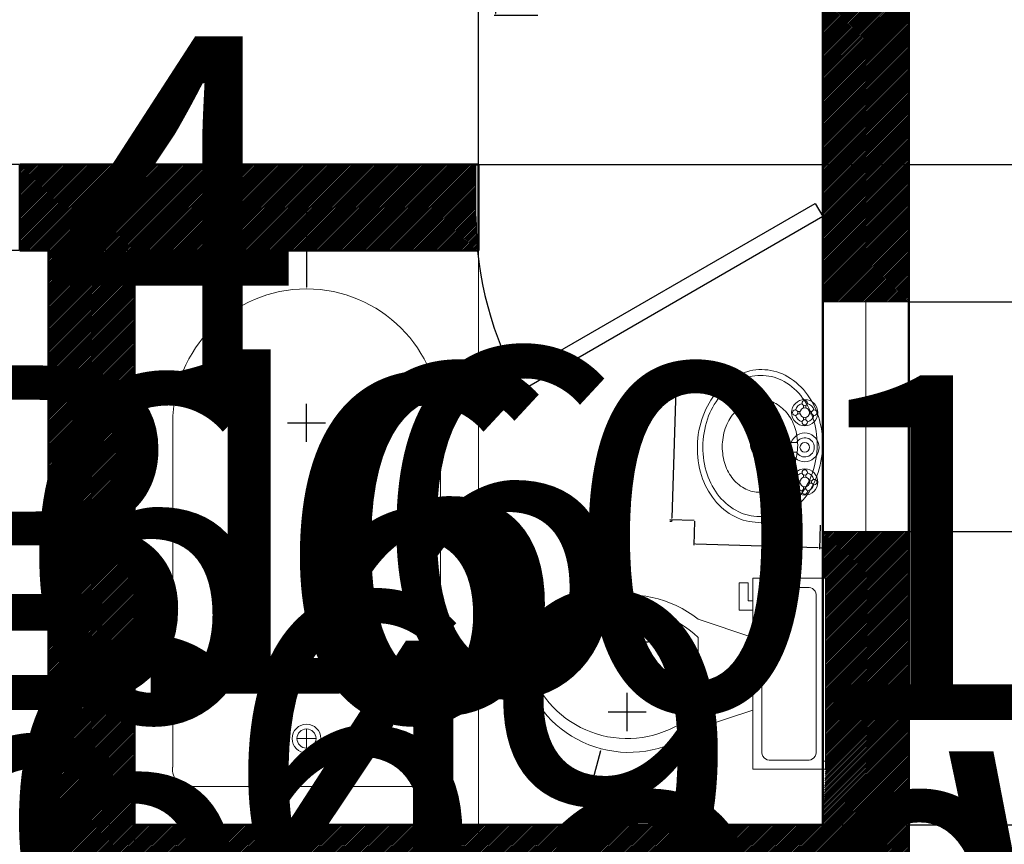
# Model space of a CAD drawing. Units: inches. Extents: x 1173 to 2157, y 515 to 1129.
# Tile 8 of 13: x 1578 to 1681, y 862 to 948. Entities that reach past the tile are written whole.
import ezdxf

# ---------------------------------------------------------------- set-up
doc = ezdxf.new("R2010")
doc.units = ezdxf.units.IN
doc.header["$MEASUREMENT"] = 0
for name, color, linetype, lineweight in [('A-ANNO-DIMS', 2, 'Continuous', 18), ('A-DOOR', 3, 'Continuous', 25), ('A-FLOR-FIXT', 9, 'Continuous', 18), ('A-GLAZ', 4, 'Continuous', 18), ('A-WALL', 7, 'Continuous', 50)]:
    doc.layers.add(name, color=color, linetype=linetype, lineweight=lineweight)
doc.layers.add('A-WALL-PATT', color=22, linetype='Continuous', lineweight=13, true_color=0xca4b0c)
doc.styles.get("Standard").update_dxf_attribs({"font": 'arial.ttf'})
doc.dimstyles.get("Standard").update_dxf_attribs({"dimtxt": 36, "dimasz": 0.18, "dimexe": 0.18, "dimexo": 0.0625, "dimgap": 0.09, "dimtad": 0, "dimtih": 1, "dimtoh": 1, "dimdec": 0, "dimrnd": 72, "dimzin": 0, "dimdsep": 46, "dimlunit": 3, "dimtxsty": 'Standard', "dimcen": 2, "dimadec": 0, "dimazin": 0, "dimtfac": 1, "dimtdec": 0, "dimtofl": 0, "dimtmove": 0, "dimatfit": 3, "dimfxl": 1, "dimtolj": 1, "dimtzin": 0, "dimarcsym": 0})

# ---------------------------------------------------------------- blocks, each defined once
blk = doc.blocks.new('*U23')
for p, q in [((-40, 0), (-40, 6)), ((0, 0), (0, 6))]:
    blk.add_line(p, q)
blk.add_lwpolyline([(0, 0), (-34.64, -20), (-35.52, -18.48), (-0.88, 1.52)], close=True)
blk.add_arc((0, 0), 40, 180, 210)
blk = doc.blocks.new('Bath Tub - 26 x 60 in.')
for p, q in [((9, -17), (9, -19)), ((8, -18), (10, -18))]:
    blk.add_line(p, q)
blk.add_lwpolyline([(0, -36), (0, 0), (60, 0), (60, -36)], close=True)
for points in [[(6, -4), (42, -4)], [(4, -30), (4, -6)], [(42, -32), (6, -32)]]:
    blk.add_lwpolyline(points)
for radius in [1.5, 1]:
    blk.add_circle((9, -18), radius)
for centre, radius, start, end in [((5.75, -5.75), 1.77, 81.8699, 188.1301), ((42, -18), 14, 270, 90), ((5.75, -30.25), 1.77, 171.8699, 278.1301)]:
    blk.add_arc(centre, radius, start, end)
blk = doc.blocks.new('Toilet - top')
for p, q in [((9.5, -6), (9.5, -2)), ((-10, -8.5), (-8, -8.5)), ((-10, -9.5), (-10, -8.5)), ((-8, -8.5), (-8, -8)), ((-7, -8), (-7, -9.5)), ((-4, -8), (-6, -14)), ((4, -8), (6, -14)), ((-7, -9.5), (-10, -9.5)), ((4, -14), (-4, -14))]:
    blk.add_line(p, q)
blk.add_lwpolyline([(10.5, -8), (10.5, 0), (-10.5, 0), (-10.5, -8)], close=True)
for points in [[(8.5, -1), (-8.5, -1)], [(-9.5, -2), (-9.5, -6)], [(-8.5, -7), (8.5, -7)]]:
    blk.add_lwpolyline(points)
for centre, radius, start, end in [((-8.62, -1.88), 0.884, 81.8699, 188.1301), ((8.62, -1.88), 0.884, 351.8699, 98.1301), ((-8.62, -6.12), 0.884, 171.8699, 278.1301), ((8.62, -6.12), 0.884, 261.8699, 8.1301), ((3.52, -21.58), 12.17, 141.4691, 247.9714), ((4.2, -21.82), 11.33, 136.3677, 238.9468), ((-3.52, -21.58), 12.17, 292.0284, 38.5307), ((-4.2, -21.82), 11.33, 301.053, 43.6321), ((0, -27.88), 4, 245.7318, 294.2682), ((0, -29), 4, 254.8605, 285.1395)]:
    blk.add_arc(centre, radius, start, end)
blk = doc.blocks.new('Sink - Oval top')
for p, q in [((-1, 0), (1, 0)), ((0, 1), (0, -1))]:
    blk.add_line(p, q)
for points in [[(-12.23, 0.39, 0.117634), (-11.46, -3.36, 0.104469), (-8.88, -6.8, 0.090016), (-5.08, -9.07, 0.08192), (-0.32, -10.02, 0.08192), (4.49, -9.38, 0.090016), (8.42, -7.36, 0.104469), (11.22, -4.09, 0.117634), (12.23, -0.39, 0.117634), (11.46, 3.36, 0.104469), (8.88, 6.8, 0.090016), (5.08, 9.07, 0.08192), (0.32, 10.02, 0.08192), (-4.49, 9.38, 0.090016), (-8.42, 7.36, 0.104469), (-11.22, 4.09, 0.117634)], [(-11.29, 0.16, 0.118622), (-10.52, -3.25, 0.104678), (-8.07, -6.36, 0.089562), (-4.54, -8.37, 0.081185), (-0.13, -9.15, 0.081185), (4.3, -8.49, 0.089562), (7.89, -6.58, 0.104678), (10.42, -3.55, 0.118622), (11.29, -0.16, 0.118622), (10.52, 3.25, 0.104678), (8.07, 6.36, 0.089562), (4.54, 8.37, 0.081185), (0.13, 9.15, 0.081185), (-4.3, 8.49, 0.089562), (-7.89, 6.58, 0.104678), (-10.42, 3.55, 0.118622)], [(-7.42, 0.08, 0.118283), (-6.91, -2.17, 0.104607), (-5.29, -4.21, 0.089718), (-2.97, -5.53, 0.081436), (-0.07, -6.04, 0.081436), (2.84, -5.59, 0.089718), (5.2, -4.33, 0.104607), (6.86, -2.32, 0.118283), (7.42, -0.08, 0.118283), (6.91, 2.17, 0.104607), (5.29, 4.21, 0.089718), (2.97, 5.53, 0.081436), (0.07, 6.04, 0.081436), (-2.84, 5.59, 0.089718), (-5.2, 4.33, 0.104607), (-6.86, 2.32, 0.118283)]]:
    blk.add_lwpolyline(points, format="xyb", close=True)
for radius in [1.5, 1]:
    blk.add_circle((0, 0), radius)
blk = doc.blocks.new('Faucet - Bathroom top')
for p, q in [((-4.107, 0.125), (-4.375, 0.125)), ((-3.75, 0.4788), (-3.75, 0.75)), ((-3.5, 0.482), (-3.5, 0.75)), ((-3.1461, 0.125), (-2.875, 0.125)), ((3.143, 0.125), (2.875, 0.125)), ((3.5, 0.4788), (3.5, 0.75)), ((3.75, 0.482), (3.75, 0.75)), ((4.1039, 0.125), (4.375, 0.125)), ((-4.1039, -0.125), (-4.375, -0.125)), ((-3.75, -0.4821), (-3.75, -0.75)), ((-3.5, -0.4789), (-3.5, -0.75)), ((-3.143, -0.125), (-2.875, -0.125)), ((-0.5, -0.8639), (-0.5, -4.5)), ((0.5, -4.5), (0.5, -0.8631)), ((3.1461, -0.125), (2.875, -0.125)), ((3.5, -0.4821), (3.5, -0.75)), ((3.75, -0.4789), (3.75, -0.75)), ((4.107, -0.125), (4.375, -0.125))]:
    blk.add_line(p, q)
for centre, radius in [((-3.625, 0), 1.375), ((-3.625, 1), 0.2795), ((3.625, 0), 1.375), ((3.625, 1), 0.2795), ((-4.625, 0), 0.2795), ((-3.625, 0), 0.5), ((-2.625, 0), 0.2795), ((0, 0), 0.5), ((2.625, 0), 0.2795), ((3.625, 0), 0.5), ((4.625, 0), 0.2795), ((-3.625, -1), 0.2795), ((3.625, -1), 0.2795)]:
    blk.add_circle(centre, radius)
for centre, radius, start, end in [((0, 0), 1.5, 289.6514, 250.3603), ((-3.625, 0), 1, 105.2407, 164.2093), ((-3.625, 0), 1, 16.44125, 74.07887), ((0, 0), 1, 300.3431, 239.7554), ((3.625, 0), 1, 106.12, 164.0884), ((3.625, 0), 1, 16.23422, 73.90469), ((-3.625, 0), 1, 196.2342, 253.9047), ((-3.625, 0), 1, 286.12, 344.0884), ((3.625, 0), 1, 196.4413, 254.0789), ((3.625, 0), 1, 285.2407, 344.2093), ((0, -4.5), 0.5, 180, 0)]:
    blk.add_arc(centre, radius, start, end)
blk = doc.blocks.new('*D28')
at = {"layer": 'A-ANNO-DIMS', "color": 0, "lineweight": -2, "transparency": 16777216}
for p, q in [((1581.66, 978.31), (1581.66, 966.19)), ((1661.66, 978.31), (1661.66, 966.19)), ((1581.84, 966.37), (1661.48, 966.37)), ((1661.66, 966.37), (1661.84, 966.37))]:
    blk.add_line(p, q, dxfattribs=at)
at = {"layer": 'A-ANNO-DIMS', "color": 0, "transparency": 16777216}
for points in [[(1581.84, 966.4), (1581.84, 966.34), (1581.66, 966.37)], [(1661.48, 966.4), (1661.48, 966.34), (1661.66, 966.37)]]:
    blk.add_solid(points, dxfattribs=at)
at = {"layer": 'Defpoints', "color": 0, "transparency": 16777216}
for p in [(1581.66, 978.37), (1661.66, 978.37), (1661.66, 966.37)]:
    blk.add_point(p, dxfattribs=at)
at = {"layer": 'A-ANNO-DIMS', "color": 0, "transparency": 16777216, "insert": (1904.61, 966.37), "char_height": 36, "attachment_point": 5}
blk.add_mtext('\\A1;QUEEN BED 80 TYP.', dxfattribs=at)
blk = doc.blocks.new('*D34')
at = {"layer": 'A-ANNO-DIMS', "color": 0, "lineweight": -2, "transparency": 16777216}
for p, q in [((1631.9, 978.41), (1631.9, 982.97)), ((1632.08, 982.79), (1661.32, 982.79)), ((1661.5, 978.41), (1661.5, 982.97)), ((1661.5, 982.79), (1661.68, 982.79))]:
    blk.add_line(p, q, dxfattribs=at)
at = {"layer": 'A-ANNO-DIMS', "color": 0, "transparency": 16777216}
for points in [[(1632.08, 982.82), (1632.08, 982.76), (1631.9, 982.79)], [(1661.32, 982.82), (1661.32, 982.76), (1661.5, 982.79)]]:
    blk.add_solid(points, dxfattribs=at)
at = {"layer": 'Defpoints', "color": 0, "transparency": 16777216}
for p in [(1661.5, 982.79), (1631.9, 978.35), (1661.5, 978.35)]:
    blk.add_point(p, dxfattribs=at)
at = {"layer": 'A-ANNO-DIMS', "color": 0, "transparency": 16777216, "insert": (1918.96, 982.79), "char_height": 36, "attachment_point": 5}
blk.add_mtext('\\A1;NIGHTSTAND 30 TYP.', dxfattribs=at)
blk = doc.blocks.new('*D35')
at = {"layer": 'A-ANNO-DIMS', "color": 0, "lineweight": -2, "transparency": 16777216}
for p, q in [((1631.84, 978.35), (1627.28, 978.35)), ((1627.46, 978.35), (1627.46, 978.53)), ((1627.46, 978.53), (1627.64, 978.53)), ((1627.46, 949.05), (1627.46, 978.17)), ((1631.84, 948.87), (1627.28, 948.87))]:
    blk.add_line(p, q, dxfattribs=at)
at = {"layer": 'A-ANNO-DIMS', "color": 0, "transparency": 16777216}
for points in [[(1627.43, 978.17), (1627.49, 978.17), (1627.46, 978.35)], [(1627.43, 949.05), (1627.49, 949.05), (1627.46, 948.87)]]:
    blk.add_solid(points, dxfattribs=at)
at = {"layer": 'Defpoints', "color": 0, "transparency": 16777216}
for p in [(1627.46, 978.35), (1631.9, 978.35), (1631.9, 948.87)]:
    blk.add_point(p, dxfattribs=at)
at = {"layer": 'A-ANNO-DIMS', "color": 0, "transparency": 16777216, "insert": (1715.66, 978.53), "char_height": 36, "attachment_point": 5}
blk.add_mtext('\\A1;29 TYP.', dxfattribs=at)
blk = doc.blocks.new('*D36')
at = {"layer": 'A-ANNO-DIMS', "color": 0, "lineweight": -2, "transparency": 16777216}
for p, q in [((1497.87, 905.02), (1487.37, 905.02)), ((1487.55, 904.84), (1487.55, 889.09)), ((1487.55, 835.93), (1487.55, 851.68)), ((1497.87, 835.75), (1487.37, 835.75))]:
    blk.add_line(p, q, dxfattribs=at)
at = {"layer": 'A-ANNO-DIMS', "color": 0, "transparency": 16777216}
for points in [[(1487.52, 904.84), (1487.58, 904.84), (1487.55, 905.02)], [(1487.52, 835.93), (1487.58, 835.93), (1487.55, 835.75)]]:
    blk.add_solid(points, dxfattribs=at)
at = {"layer": 'Defpoints', "color": 0, "transparency": 16777216}
for p in [(1497.94, 905.02), (1487.55, 835.75), (1497.94, 835.75)]:
    blk.add_point(p, dxfattribs=at)
at = {"layer": 'A-ANNO-DIMS', "color": 0, "transparency": 16777216, "insert": (1487.55, 870.38), "char_height": 36, "attachment_point": 5}
blk.add_mtext('\\A1;DINING SET 69', dxfattribs=at)
blk = doc.blocks.new('*D38')
at = {"layer": 'A-ANNO-DIMS', "color": 0, "lineweight": -2, "transparency": 16777216}
for p, q in [((1471.69, 862.7), (1478.04, 862.7)), ((1477.86, 862.52), (1477.86, 860.65)), ((1477.86, 821.35), (1477.86, 823.22)), ((1471.69, 821.17), (1478.04, 821.17))]:
    blk.add_line(p, q, dxfattribs=at)
at = {"layer": 'A-ANNO-DIMS', "color": 0, "transparency": 16777216}
for points in [[(1477.83, 862.52), (1477.89, 862.52), (1477.86, 862.7)], [(1477.83, 821.35), (1477.89, 821.35), (1477.86, 821.17)]]:
    blk.add_solid(points, dxfattribs=at)
at = {"layer": 'Defpoints', "color": 0, "transparency": 16777216}
for p in [(1471.63, 862.7), (1477.86, 862.7), (1471.63, 821.17)]:
    blk.add_point(p, dxfattribs=at)
at = {"layer": 'A-ANNO-DIMS', "color": 0, "transparency": 16777216, "insert": (1477.86, 841.93), "char_height": 36, "attachment_point": 5}
blk.add_mtext('\\A1;COFFEE TABLE 42', dxfattribs=at)
blk = doc.blocks.new('*D40')
at = {"layer": 'A-ANNO-DIMS', "color": 0, "lineweight": -2, "transparency": 16777216}
for p, q in [((1422.73, 872.86), (1431.84, 872.86)), ((1431.66, 872.68), (1431.66, 861.58)), ((1431.66, 813.04), (1431.66, 824.15)), ((1422.73, 812.86), (1431.84, 812.86))]:
    blk.add_line(p, q, dxfattribs=at)
at = {"layer": 'A-ANNO-DIMS', "color": 0, "transparency": 16777216}
for points in [[(1431.63, 872.68), (1431.69, 872.68), (1431.66, 872.86)], [(1431.63, 813.04), (1431.69, 813.04), (1431.66, 812.86)]]:
    blk.add_solid(points, dxfattribs=at)
at = {"layer": 'Defpoints', "color": 0, "transparency": 16777216}
for p in [(1422.66, 872.86), (1431.66, 872.86), (1422.66, 812.86)]:
    blk.add_point(p, dxfattribs=at)
at = {"layer": 'A-ANNO-DIMS', "color": 0, "transparency": 16777216, "insert": (1431.66, 842.86), "char_height": 36, "attachment_point": 5}
blk.add_mtext('\\A1;LOVESEAT 60', dxfattribs=at)
blk = doc.blocks.new('*D44')
at = {"layer": 'A-ANNO-DIMS', "color": 0, "lineweight": -2, "transparency": 16777216}
for p, q in [((1630.26, 849.3), (1630.26, 854.13)), ((1630.44, 853.95), (1661.48, 853.95)), ((1661.66, 849.3), (1661.66, 854.13)), ((1661.66, 853.95), (1661.84, 853.95))]:
    blk.add_line(p, q, dxfattribs=at)
at = {"layer": 'A-ANNO-DIMS', "color": 0, "transparency": 16777216}
for points in [[(1630.44, 853.98), (1630.44, 853.92), (1630.26, 853.95)], [(1661.48, 853.98), (1661.48, 853.92), (1661.66, 853.95)]]:
    blk.add_solid(points, dxfattribs=at)
at = {"layer": 'Defpoints', "color": 0, "transparency": 16777216}
for p in [(1661.66, 853.95), (1630.26, 849.24), (1661.66, 849.24)]:
    blk.add_point(p, dxfattribs=at)
at = {"layer": 'A-ANNO-DIMS', "color": 0, "transparency": 16777216, "insert": (1799.17, 853.95), "char_height": 36, "attachment_point": 5}
blk.add_mtext('\\A1;WC 31 TYP.', dxfattribs=at)
blk = doc.blocks.new('*D45')
at = {"layer": 'A-ANNO-DIMS', "color": 0, "lineweight": -2, "transparency": 16777216}
for p, q in [((1630.2, 849.24), (1625.37, 849.24)), ((1625.55, 849.24), (1625.55, 849.42)), ((1625.55, 849.42), (1625.73, 849.42)), ((1625.55, 829.46), (1625.55, 849.06)), ((1630.2, 829.28), (1625.37, 829.28))]:
    blk.add_line(p, q, dxfattribs=at)
at = {"layer": 'A-ANNO-DIMS', "color": 0, "transparency": 16777216}
for points in [[(1625.52, 849.06), (1625.58, 849.06), (1625.55, 849.24)], [(1625.52, 829.46), (1625.58, 829.46), (1625.55, 829.28)]]:
    blk.add_solid(points, dxfattribs=at)
at = {"layer": 'Defpoints', "color": 0, "transparency": 16777216}
for p in [(1625.55, 849.24), (1630.26, 849.24), (1630.26, 829.28)]:
    blk.add_point(p, dxfattribs=at)
at = {"layer": 'A-ANNO-DIMS', "color": 0, "transparency": 16777216, "insert": (1713.74, 849.42), "char_height": 36, "attachment_point": 5}
blk.add_mtext('\\A1;20 TYP.', dxfattribs=at)
blk = doc.blocks.new('*D46')
at = {"layer": 'A-ANNO-DIMS', "color": 0, "lineweight": -2, "transparency": 16777216}
for p, q in [((1646.37, 911.98), (1645.86, 896.32)), ((1648.72, 912.09), (1646.2, 912.17)), ((1645.85, 895.96), (1645.67, 895.96)), ((1648.2, 896.07), (1645.68, 896.15)), ((1645.86, 896.14), (1645.85, 895.96))]:
    blk.add_line(p, q, dxfattribs=at)
at = {"layer": 'A-ANNO-DIMS', "color": 0, "transparency": 16777216}
for points in [[(1646.34, 911.99), (1646.4, 911.98), (1646.38, 912.16)], [(1645.83, 896.32), (1645.89, 896.32), (1645.86, 896.14)]]:
    blk.add_solid(points, dxfattribs=at)
at = {"layer": 'Defpoints', "color": 0, "transparency": 16777216}
for p in [(1648.78, 912.09), (1645.86, 896.14), (1648.26, 896.06)]:
    blk.add_point(p, dxfattribs=at)
at = {"layer": 'A-ANNO-DIMS', "color": 0, "transparency": 16777216, "insert": (1538.16, 895.96), "char_height": 36, "attachment_point": 5}
blk.add_mtext('\\A1;BASIN 16', dxfattribs=at)
blk = doc.blocks.new('*D47')
at = {"layer": 'A-ANNO-DIMS', "color": 0, "lineweight": -2, "transparency": 16777216}
for p, q in [((1648.26, 896), (1648.18, 893.48)), ((1661.4, 895.58), (1661.32, 893.06)), ((1648.36, 893.65), (1661.15, 893.24)), ((1661.33, 893.24), (1661.51, 893.23))]:
    blk.add_line(p, q, dxfattribs=at)
at = {"layer": 'A-ANNO-DIMS', "color": 0, "transparency": 16777216}
for points in [[(1648.37, 893.68), (1648.36, 893.62), (1648.18, 893.66)], [(1661.15, 893.27), (1661.15, 893.21), (1661.33, 893.24)]]:
    blk.add_solid(points, dxfattribs=at)
at = {"layer": 'Defpoints', "color": 0, "transparency": 16777216}
for p in [(1648.26, 896.06), (1661.4, 895.64), (1661.33, 893.24)]:
    blk.add_point(p, dxfattribs=at)
at = {"layer": 'A-ANNO-DIMS', "color": 0, "transparency": 16777216, "insert": (1685.69, 893.23), "char_height": 36, "attachment_point": 5}
blk.add_mtext('\\A1;13', dxfattribs=at)
blk = doc.blocks.new('*D48')
at = {"layer": 'A-ANNO-DIMS', "color": 0, "lineweight": -2, "transparency": 16777216}
for p, q in [((1592.53, 826.46), (1592.35, 826.47)), ((1592.38, 821.85), (1592.54, 826.64)), ((1623.53, 825.46), (1592.71, 826.46)), ((1623.56, 820.84), (1623.71, 825.64))]:
    blk.add_line(p, q, dxfattribs=at)
at = {"layer": 'A-ANNO-DIMS', "color": 0, "transparency": 16777216}
for points in [[(1592.71, 826.49), (1592.71, 826.43), (1592.53, 826.46)], [(1623.53, 825.49), (1623.53, 825.43), (1623.71, 825.46)]]:
    blk.add_solid(points, dxfattribs=at)
at = {"layer": 'Defpoints', "color": 0, "transparency": 16777216}
for p in [(1592.53, 826.46), (1592.38, 821.79), (1623.56, 820.78)]:
    blk.add_point(p, dxfattribs=at)
at = {"layer": 'A-ANNO-DIMS', "color": 0, "transparency": 16777216, "insert": (1488.3, 826.47), "char_height": 36, "attachment_point": 5}
blk.add_mtext('\\A1;BASIN 31', dxfattribs=at)
blk = doc.blocks.new('*D50')
at = {"layer": 'A-ANNO-DIMS', "color": 0, "lineweight": -2, "transparency": 16777216}
for p, q in [((1603.33, 798.21), (1603.33, 796.59)), ((1613.33, 798.21), (1613.33, 796.59)), ((1603.33, 796.77), (1603.15, 796.77)), ((1613.15, 796.77), (1603.51, 796.77))]:
    blk.add_line(p, q, dxfattribs=at)
at = {"layer": 'A-ANNO-DIMS', "color": 0, "transparency": 16777216}
for points in [[(1603.51, 796.8), (1603.51, 796.74), (1603.33, 796.77)], [(1613.15, 796.8), (1613.15, 796.74), (1613.33, 796.77)]]:
    blk.add_solid(points, dxfattribs=at)
at = {"layer": 'Defpoints', "color": 0, "transparency": 16777216}
for p in [(1603.33, 798.27), (1613.33, 798.27), (1603.33, 796.77)]:
    blk.add_point(p, dxfattribs=at)
at = {"layer": 'A-ANNO-DIMS', "color": 0, "transparency": 16777216, "insert": (1377.9, 796.77), "char_height": 36, "attachment_point": 5}
blk.add_mtext('\\A1;BASIN TAP 10 TYP.', dxfattribs=at)
blk = doc.blocks.new('*D52')
at = {"layer": 'A-ANNO-DIMS', "color": 0, "lineweight": -2, "transparency": 16777216}
for p, q in [((1589.6, 924.28), (1580.48, 924.28)), ((1580.66, 924.1), (1580.66, 912.75)), ((1580.66, 864.46), (1580.66, 875.81)), ((1589.6, 864.28), (1580.48, 864.28))]:
    blk.add_line(p, q, dxfattribs=at)
at = {"layer": 'A-ANNO-DIMS', "color": 0, "transparency": 16777216}
for points in [[(1580.63, 924.1), (1580.69, 924.1), (1580.66, 924.28)], [(1580.63, 864.46), (1580.69, 864.46), (1580.66, 864.28)]]:
    blk.add_solid(points, dxfattribs=at)
at = {"layer": 'Defpoints', "color": 0, "transparency": 16777216}
for p in [(1580.66, 924.28), (1589.66, 924.28), (1589.66, 864.28)]:
    blk.add_point(p, dxfattribs=at)
at = {"layer": 'A-ANNO-DIMS', "color": 0, "transparency": 16777216, "insert": (1580.66, 894.28), "char_height": 36, "attachment_point": 5}
blk.add_mtext('\\A1;TUB 60', dxfattribs=at)
blk = doc.blocks.new('*D53')
at = {"layer": 'A-ANNO-DIMS', "color": 0, "lineweight": -2, "transparency": 16777216}
for p, q in [((1589.66, 864.22), (1589.66, 855.1)), ((1625.66, 864.22), (1625.66, 855.1)), ((1589.66, 855.28), (1589.48, 855.28)), ((1625.48, 855.28), (1589.84, 855.28))]:
    blk.add_line(p, q, dxfattribs=at)
at = {"layer": 'A-ANNO-DIMS', "color": 0, "transparency": 16777216}
for points in [[(1589.84, 855.31), (1589.84, 855.25), (1589.66, 855.28)], [(1625.48, 855.31), (1625.48, 855.25), (1625.66, 855.28)]]:
    blk.add_solid(points, dxfattribs=at)
at = {"layer": 'Defpoints', "color": 0, "transparency": 16777216}
for p in [(1589.66, 864.28), (1625.66, 864.28), (1589.66, 855.28)]:
    blk.add_point(p, dxfattribs=at)
at = {"layer": 'A-ANNO-DIMS', "color": 0, "transparency": 16777216, "insert": (1563.63, 855.28), "char_height": 36, "attachment_point": 5}
blk.add_mtext('\\A1;36', dxfattribs=at)
blk = doc.blocks.new('*D54')
at = {"layer": 'A-ANNO-DIMS', "color": 0, "lineweight": -2, "transparency": 16777216}
for p, q in [((1496.35, 1005.18), (1488.93, 1005.18)), ((1489.11, 1005), (1489.11, 999.54)), ((1489.11, 956.65), (1489.11, 962.11)), ((1496.35, 956.47), (1488.93, 956.47))]:
    blk.add_line(p, q, dxfattribs=at)
at = {"layer": 'A-ANNO-DIMS', "color": 0, "transparency": 16777216}
for points in [[(1489.08, 1005), (1489.14, 1005), (1489.11, 1005.18)], [(1489.08, 956.65), (1489.14, 956.65), (1489.11, 956.47)]]:
    blk.add_solid(points, dxfattribs=at)
at = {"layer": 'Defpoints', "color": 0, "transparency": 16777216}
for p in [(1496.42, 1005.18), (1489.11, 956.47), (1496.42, 956.47)]:
    blk.add_point(p, dxfattribs=at)
at = {"layer": 'A-ANNO-DIMS', "color": 0, "transparency": 16777216, "insert": (1489.11, 980.83), "char_height": 36, "attachment_point": 5}
blk.add_mtext('\\A1;WORK TABLE 49', dxfattribs=at)
blk = doc.blocks.new('*D60')
at = {"layer": 'A-ANNO-DIMS', "color": 0, "lineweight": -2, "transparency": 16777216}
for p, q in [((1396.06, 971.62), (1390.55, 971.62)), ((1390.73, 971.62), (1390.73, 971.8)), ((1390.73, 971.8), (1390.91, 971.8)), ((1390.73, 935.8), (1390.73, 971.44)), ((1396.06, 935.62), (1390.55, 935.62))]:
    blk.add_line(p, q, dxfattribs=at)
at = {"layer": 'A-ANNO-DIMS', "color": 0, "transparency": 16777216}
for points in [[(1390.7, 971.44), (1390.76, 971.44), (1390.73, 971.62)], [(1390.7, 935.8), (1390.76, 935.8), (1390.73, 935.62)]]:
    blk.add_solid(points, dxfattribs=at)
at = {"layer": 'Defpoints', "color": 0, "transparency": 16777216}
for p in [(1390.73, 971.62), (1396.13, 971.62), (1396.13, 935.62)]:
    blk.add_point(p, dxfattribs=at)
at = {"layer": 'A-ANNO-DIMS', "color": 0, "transparency": 16777216, "insert": (1517.73, 971.8), "char_height": 36, "attachment_point": 5}
blk.add_mtext('\\A1;FRIDGE 36', dxfattribs=at)
blk = doc.blocks.new('*D90')
at = {"layer": 'A-ANNO-DIMS', "color": 0, "lineweight": -2, "transparency": 16777216}
for p, q in [((1661.73, 1044.28), (1696.15, 1044.28)), ((1695.97, 1044.1), (1695.97, 1006.94)), ((1695.97, 933.46), (1695.97, 970.62)), ((1625.73, 933.28), (1696.15, 933.28))]:
    blk.add_line(p, q, dxfattribs=at)
at = {"layer": 'A-ANNO-DIMS', "color": 0, "transparency": 16777216}
for points in [[(1695.94, 1044.1), (1696, 1044.1), (1695.97, 1044.28)], [(1695.94, 933.46), (1696, 933.46), (1695.97, 933.28)]]:
    blk.add_solid(points, dxfattribs=at)
at = {"layer": 'Defpoints', "color": 0, "transparency": 16777216}
for p in [(1661.66, 1044.28), (1625.66, 933.28), (1695.97, 933.28)]:
    blk.add_point(p, dxfattribs=at)
at = {"layer": 'A-ANNO-DIMS', "color": 0, "transparency": 16777216, "insert": (1695.97, 988.78), "char_height": 36, "attachment_point": 5}
blk.add_mtext('\\A1;111', dxfattribs=at)
blk = doc.blocks.new('*D94')
at = {"layer": 'A-ANNO-DIMS', "color": 0, "lineweight": -2, "transparency": 16777216}
for p, q in [((1577.6, 933.28), (1552.18, 933.28)), ((1552.36, 933.28), (1552.36, 933.46)), ((1552.36, 933.46), (1552.54, 933.46)), ((1552.36, 924.46), (1552.36, 933.1)), ((1577.6, 924.28), (1552.18, 924.28))]:
    blk.add_line(p, q, dxfattribs=at)
at = {"layer": 'A-ANNO-DIMS', "color": 0, "transparency": 16777216}
for points in [[(1552.33, 933.1), (1552.39, 933.1), (1552.36, 933.28)], [(1552.33, 924.46), (1552.39, 924.46), (1552.36, 924.28)]]:
    blk.add_solid(points, dxfattribs=at)
at = {"layer": 'Defpoints', "color": 0, "transparency": 16777216}
for p in [(1552.36, 933.28), (1577.66, 933.28), (1577.66, 924.28)]:
    blk.add_point(p, dxfattribs=at)
at = {"layer": 'A-ANNO-DIMS', "color": 0, "transparency": 16777216, "insert": (1564.47, 933.46), "char_height": 36, "attachment_point": 5}
blk.add_mtext('\\A1;9', dxfattribs=at)
blk = doc.blocks.new('*D97')
at = {"layer": 'A-ANNO-DIMS', "color": 0, "lineweight": -2, "transparency": 16777216}
for p, q in [((1580.6, 855.28), (1354.18, 855.28)), ((1354.36, 855.28), (1354.36, 855.46)), ((1354.36, 855.46), (1354.54, 855.46)), ((1354.36, 819.46), (1354.36, 855.1)), ((1580.6, 819.28), (1354.18, 819.28))]:
    blk.add_line(p, q, dxfattribs=at)
at = {"layer": 'A-ANNO-DIMS', "color": 0, "transparency": 16777216}
for points in [[(1354.33, 855.1), (1354.39, 855.1), (1354.36, 855.28)], [(1354.33, 819.46), (1354.39, 819.46), (1354.36, 819.28)]]:
    blk.add_solid(points, dxfattribs=at)
at = {"layer": 'Defpoints', "color": 0, "transparency": 16777216}
for p in [(1354.36, 855.28), (1580.66, 855.28), (1580.66, 819.28)]:
    blk.add_point(p, dxfattribs=at)
at = {"layer": 'A-ANNO-DIMS', "color": 0, "transparency": 16777216, "insert": (1380.39, 855.46), "char_height": 36, "attachment_point": 5}
blk.add_mtext('\\A1;36', dxfattribs=at)
blk = doc.blocks.new('*D98')
at = {"layer": 'A-ANNO-DIMS', "color": 0, "lineweight": -2, "transparency": 16777216}
for p, q in [((1625.66, 924.34), (1625.66, 1078.79)), ((1625.84, 1078.61), (1661.48, 1078.61)), ((1661.66, 924.34), (1661.66, 1078.79)), ((1661.66, 1078.61), (1661.84, 1078.61))]:
    blk.add_line(p, q, dxfattribs=at)
at = {"layer": 'A-ANNO-DIMS', "color": 0, "transparency": 16777216}
for points in [[(1625.84, 1078.64), (1625.84, 1078.58), (1625.66, 1078.61)], [(1661.48, 1078.64), (1661.48, 1078.58), (1661.66, 1078.61)]]:
    blk.add_solid(points, dxfattribs=at)
at = {"layer": 'Defpoints', "color": 0, "transparency": 16777216}
for p in [(1661.66, 1078.61), (1625.66, 924.28), (1661.66, 924.28)]:
    blk.add_point(p, dxfattribs=at)
at = {"layer": 'A-ANNO-DIMS', "color": 0, "transparency": 16777216, "insert": (1687.69, 1078.61), "char_height": 36, "attachment_point": 5}
blk.add_mtext('\\A1;36', dxfattribs=at)
blk = doc.blocks.new('*D99')
at = {"layer": 'A-ANNO-DIMS', "color": 0, "lineweight": -2, "transparency": 16777216}
for p, q in [((1670.73, 918.92), (1696.15, 918.92)), ((1695.97, 918.92), (1695.97, 919.1)), ((1695.97, 919.1), (1696.15, 919.1)), ((1695.97, 895.1), (1695.97, 918.74)), ((1670.73, 894.92), (1696.15, 894.92))]:
    blk.add_line(p, q, dxfattribs=at)
at = {"layer": 'A-ANNO-DIMS', "color": 0, "transparency": 16777216}
for points in [[(1695.94, 918.74), (1696, 918.74), (1695.97, 918.92)], [(1695.94, 895.1), (1696, 895.1), (1695.97, 894.92)]]:
    blk.add_solid(points, dxfattribs=at)
at = {"layer": 'Defpoints', "color": 0, "transparency": 16777216}
for p in [(1670.66, 918.92), (1695.97, 918.92), (1670.66, 894.92)]:
    blk.add_point(p, dxfattribs=at)
at = {"layer": 'A-ANNO-DIMS', "color": 0, "transparency": 16777216, "insert": (1722.25, 919.1), "char_height": 36, "attachment_point": 5}
blk.add_mtext('\\A1;24', dxfattribs=at)
blk = doc.blocks.new('*D100')
at = {"layer": 'A-ANNO-DIMS', "color": 0, "lineweight": -2, "transparency": 16777216}
for p, q in [((1695.97, 894.92), (1695.97, 895.1)), ((1695.97, 895.1), (1696.15, 895.1)), ((1661.73, 894.92), (1696.15, 894.92)), ((1695.97, 864.46), (1695.97, 894.74)), ((1661.73, 864.28), (1696.15, 864.28))]:
    blk.add_line(p, q, dxfattribs=at)
at = {"layer": 'A-ANNO-DIMS', "color": 0, "transparency": 16777216}
for points in [[(1695.94, 894.74), (1696, 894.74), (1695.97, 894.92)], [(1695.94, 864.46), (1696, 864.46), (1695.97, 864.28)]]:
    blk.add_solid(points, dxfattribs=at)
at = {"layer": 'Defpoints', "color": 0, "transparency": 16777216}
for p in [(1661.66, 894.92), (1695.97, 894.92), (1661.66, 864.28)]:
    blk.add_point(p, dxfattribs=at)
at = {"layer": 'A-ANNO-DIMS', "color": 0, "transparency": 16777216, "insert": (1771.08, 895.1), "char_height": 36, "attachment_point": 5}
blk.add_mtext('\\A1;30.635', dxfattribs=at)
blk = doc.blocks.new('*D102')
at = {"layer": 'A-ANNO-DIMS', "color": 0, "lineweight": -2, "transparency": 16777216}
for p, q in [((1661.73, 855.28), (1696.15, 855.28)), ((1695.97, 855.28), (1695.97, 855.46)), ((1695.97, 855.46), (1696.15, 855.46)), ((1695.97, 826.74), (1695.97, 855.1)), ((1670.73, 826.56), (1696.15, 826.56))]:
    blk.add_line(p, q, dxfattribs=at)
at = {"layer": 'A-ANNO-DIMS', "color": 0, "transparency": 16777216}
for points in [[(1695.94, 855.1), (1696, 855.1), (1695.97, 855.28)], [(1695.94, 826.74), (1696, 826.74), (1695.97, 826.56)]]:
    blk.add_solid(points, dxfattribs=at)
at = {"layer": 'Defpoints', "color": 0, "transparency": 16777216}
for p in [(1661.66, 855.28), (1695.97, 855.28), (1670.66, 826.56)]:
    blk.add_point(p, dxfattribs=at)
at = {"layer": 'A-ANNO-DIMS', "color": 0, "transparency": 16777216, "insert": (1757.1, 855.46), "char_height": 36, "attachment_point": 5}
blk.add_mtext('\\A1;28.72', dxfattribs=at)
blk = doc.blocks.new('*D107')
at = {"layer": 'A-ANNO-DIMS', "color": 0, "lineweight": -2, "transparency": 16777216}
for p, q in [((1607.48, 928.68), (1607.66, 928.68)), ((1607.66, 928.68), (1607.66, 920.46)), ((1607.66, 904.28), (1607.66, 908.28)), ((1605.66, 906.28), (1609.66, 906.28))]:
    blk.add_line(p, q, dxfattribs=at)
at = {"layer": 'A-ANNO-DIMS', "color": 0, "transparency": 16777216}
blk.add_solid([(1607.69, 920.46), (1607.63, 920.46), (1607.66, 920.28)], dxfattribs=at)
at = {"layer": 'Defpoints', "color": 0, "transparency": 16777216}
for p in [(1607.66, 920.28), (1607.66, 906.28)]:
    blk.add_point(p, dxfattribs=at)
at = {"layer": 'A-ANNO-DIMS', "color": 0, "transparency": 16777216, "insert": (1564.46, 928.68), "char_height": 36, "attachment_point": 5}
blk.add_mtext('\\A1;R14', dxfattribs=at)
blk = doc.blocks.new('*D108')
at = {"layer": 'A-ANNO-DIMS', "color": 0, "lineweight": -2, "transparency": 16777216}
for p, q in [((1641.43, 881.4), (1641.43, 885.4)), ((1639.43, 883.4), (1643.43, 883.4)), ((1636.72, 865.51), (1638.44, 872.04)), ((1636.54, 865.51), (1636.72, 865.51))]:
    blk.add_line(p, q, dxfattribs=at)
at = {"layer": 'A-ANNO-DIMS', "color": 0, "transparency": 16777216}
blk.add_solid([(1638.41, 872.05), (1638.47, 872.04), (1638.49, 872.22)], dxfattribs=at)
at = {"layer": 'Defpoints', "color": 0, "transparency": 16777216}
for p in [(1641.43, 883.4), (1638.49, 872.22)]:
    blk.add_point(p, dxfattribs=at)
at = {"layer": 'A-ANNO-DIMS', "color": 0, "transparency": 16777216, "insert": (1505.59, 865.51), "char_height": 36, "attachment_point": 5}
blk.add_mtext('\\A1;2X R11.564', dxfattribs=at)
blk = doc.blocks.new('*D109')
at = {"layer": 'A-ANNO-DIMS', "color": 0, "lineweight": -2, "transparency": 16777216}
for p, q in [((1638.72, 893.14), (1638.9, 893.14)), ((1638.9, 893.14), (1639.74, 886.91)), ((1641.2, 874.07), (1641.2, 878.07)), ((1639.2, 876.07), (1643.2, 876.07))]:
    blk.add_line(p, q, dxfattribs=at)
at = {"layer": 'A-ANNO-DIMS', "color": 0, "transparency": 16777216}
blk.add_solid([(1639.77, 886.92), (1639.71, 886.91), (1639.77, 886.74)], dxfattribs=at)
at = {"layer": 'Defpoints', "color": 0, "transparency": 16777216}
for p in [(1639.77, 886.74), (1641.2, 876.07)]:
    blk.add_point(p, dxfattribs=at)
at = {"layer": 'A-ANNO-DIMS', "color": 0, "transparency": 16777216, "insert": (1507.71, 893.14), "char_height": 36, "attachment_point": 5}
blk.add_mtext('\\A1;2X R10.766', dxfattribs=at)

msp = doc.modelspace()

# ---------------------------------------------------------------- hatches: boundary and pattern name
at = {"layer": 'A-WALL-PATT'}
h = msp.add_hatch(dxfattribs=at)
h.set_pattern_fill('ANSI31', color=256)
h.paths.add_polyline_path([(1388.6635, 933.2805), (1388.6635, 1044.2805), (1413.7618, 1044.2805), (1413.7618, 1053.2805), (1379.6635, 1053.2805), (1379.6635, 894.1606), (1388.6635, 894.1606), (1388.6635, 924.2805), (1472.6635, 924.2805), (1472.6635, 933.2805)])
h.paths.add_polyline_path([(1520.6635, 1044.2805), (1520.6635, 1014.7866), (1520.6635, 1005.1794), (1520.7714, 1005.1794), (1520.7714, 956.4707), (1520.6635, 924.2805), (1529.6635, 924.2805), (1529.6635, 931.4788), (1529.6635, 1044.2805), (1530.8474, 1044.2805), (1570.9543, 1044.2805), (1570.9543, 1053.2805), (1461.7618, 1053.2805), (1461.7618, 1044.2805)])
h.paths.add_polyline_path([(1618.9543, 1053.2805), (1618.9543, 1044.2805), (1661.6635, 1044.2805), (1661.6635, 1043.7367), (1661.6635, 1032.8874), (1670.6635, 1032.8874), (1670.6635, 1053.2805)])
h.paths.add_polyline_path([(1661.6635, 933.2805), (1661.6635, 927.8377), (1661.6635, 924.2805), (1661.6635, 918.9156), (1670.6635, 918.9156), (1670.6635, 984.8874), (1661.6635, 984.8874), (1661.6635, 978.3712)])
h.paths.add_polyline_path([(1670.6635, 894.9156), (1661.6635, 894.9156), (1661.6635, 890.0349), (1661.9328, 890.0349), (1661.9328, 870.079), (1661.6635, 864.2805), (1589.6635, 864.2805), (1589.6635, 924.2805), (1625.553, 924.2805, -0.02455299), (1625.3782, 927.8377), (1625.3782, 933.2805), (1577.6635, 933.2805), (1577.6635, 924.2805), (1580.6635, 924.2805), (1580.6635, 855.2805), (1586.1062, 855.2805), (1589.6635, 855.2805), (1661.6635, 855.2805), (1661.6635, 826.5597), (1670.6635, 826.5597)])
h.paths.add_polyline_path([(1670.6635, 802.5597), (1661.6635, 802.5597), (1661.6635, 795.2805), (1589.6635, 795.2805), (1589.6635, 819.17, -0.02455299), (1586.1062, 818.9952), (1580.6635, 818.9952), (1580.6635, 795.2805), (1577.6635, 795.2805), (1577.6635, 786.2805), (1661.6635, 786.2805), (1661.6635, 778.5597), (1661.6635, 742.6973), (1670.6635, 742.6973)])
h.paths.add_polyline_path([(1661.6635, 654.2805), (1625.1498, 654.2805), (1625.1498, 645.2805), (1661.3656, 645.2805), (1661.6635, 645.2805), (1661.6635, 573.2805), (1520.6635, 573.2805), (1520.6635, 564.2805), (1670.6635, 564.2805), (1670.6635, 694.6973), (1661.6635, 694.6973)])
h.paths.add_polyline_path([(1529.4367, 733.4702, -0.06854064), (1529.6635, 734.2623), (1529.6635, 795.2805), (1520.6635, 795.2805), (1520.6635, 645.2805), (1577.1498, 645.2805), (1577.1498, 654.2805), (1529.6635, 654.2805), (1529.6635, 686.5626, -0.06854064), (1529.4367, 687.3547)])
h.paths.add_polyline_path([(1379.6635, 711.2805), (1388.6635, 711.2805), (1458.7214, 711.2805), (1458.7214, 720.2805), (1410.7214, 720.2805), (1388.6635, 720.2805), (1388.6635, 745.0427), (1379.6635, 745.0427)])
h.paths.add_polyline_path([(1388.6635, 846.1606), (1379.6635, 846.1606), (1379.6635, 793.0427), (1388.6635, 793.0427)])

# ---------------------------------------------------------------- linework, layer by layer
at = {"layer": 'A-GLAZ'}
for p, q in [((1666.1635, 918.9156), (1666.1635, 894.9156)), ((1661.6635, 894.9156), (1670.6635, 894.9156))]:
    msp.add_line(p, q, dxfattribs=at)
msp.add_lwpolyline([(1661.9328, 870.9156), (1661.6635, 870.9156), (1661.6635, 918.9156), (1670.6635, 918.9156), (1670.6635, 870.9156)], dxfattribs=at)
at = {"layer": 'A-WALL'}
for p, q in [((1661.6635, 933.2805), (1661.6635, 1044.2805)), ((1625.6635, 933.2805), (1577.6635, 933.2805)), ((1577.6635, 924.2805), (1577.6635, 933.2805)), ((1625.6635, 933.2805), (1625.6635, 924.2805)), ((1661.6635, 933.2805), (1661.6635, 924.2805)), ((1580.6635, 924.2805), (1577.6635, 924.2805)), ((1580.6635, 855.2805), (1580.6635, 924.2805)), ((1625.6635, 924.2805), (1589.6635, 924.2805)), ((1589.6635, 864.2805), (1589.6635, 924.2805)), ((1661.6635, 864.2805), (1661.6635, 924.2805)), ((1661.6635, 864.2805), (1589.6635, 864.2805))]:
    msp.add_line(p, q, dxfattribs=at)
msp.add_lwpolyline([(1379.6635, 564.2805), (1670.6635, 564.2805), (1670.6635, 1053.2805), (1379.6635, 1053.2805)], close=True, dxfattribs=at)

# ---------------------------------------------------------------- block references
at = {"layer": 'A-DOOR', "xscale": 0.9071317920918195, "yscale": 0.9071317920918195, "zscale": 0.9071317920918195}
msp.add_blockref('*U23', (1661.6635, 927.8377), dxfattribs=at)
at = {"layer": 'A-FLOR-FIXT'}
for name, p, rotation in [('Bath Tub - 26 x 60 in.', (1589.6635, 864.2805), 90), ('Faucet - Bathroom top', (1659.7753, 903.7186), 270)]:
    msp.add_blockref(name, p, dxfattribs=dict(at, rotation=rotation))
for name, p, xscale, yscale, zscale, rotation in [('Sink - Oval top', (1655.0915, 903.8635), 0.6529849361859226, 0.6529849361859226, 0.6529849361859226, 268.1544699151341), ('Toilet - top', (1661.9328, 880.0569), 0.950285164574055, 0.950285164574055, 0.950285164574055, 270)]:
    msp.add_blockref(name, p, dxfattribs=dict(at, xscale=xscale, yscale=yscale, zscale=zscale, rotation=rotation))

# ---------------------------------------------------------------- dimensions: what is measured, and where the dimension line sits
at = {"layer": 'A-ANNO-DIMS'}
dim = msp.add_linear_dim(base=(1661.6635, 1078.6127), p1=(1625.6635, 924.2805), p2=(1661.6635, 924.2805), dimstyle='Standard', override={"dimdec": 0, "dimlfac": 1, "dimrnd": 0, "dimzin": 0, "dimdsep": 46, "dimlunit": 2}, dxfattribs=at)
dim.commit()
dim.dimension.update_dxf_attribs({"geometry": '*D98', "text_midpoint": (1687.6933, 1078.6127)})
for base, p1, p2, text, picture, middle in [((1661.6635, 966.3712), (1581.6634, 978.3712), (1661.6635, 978.3712), 'QUEEN BED <> TYP.', '*D28', (1904.6142, 966.3712)), ((1661.5047, 982.7919), (1631.9047, 978.3519), (1661.5047, 978.3519), 'NIGHTSTAND <> TYP.', '*D34', (1918.9562, 982.7919)), ((1661.6635, 853.9514), (1630.2601, 849.2409), (1661.6635, 849.2409), 'WC <> TYP.', '*D44', (1799.1681, 853.9514))]:
    dim = msp.add_linear_dim(base=base, p1=p1, p2=p2, text=text, dimstyle='Standard', override={"dimdec": 0, "dimlfac": 1, "dimrnd": 0, "dimzin": 0, "dimdsep": 46, "dimlunit": 2}, dxfattribs=at)
    dim.commit()
    dim.dimension.update_dxf_attribs({"geometry": picture, "text_midpoint": middle})
for base, p1, p2, angle, text, picture, middle in [((1489.1107, 956.4707), (1496.4171, 1005.1794), (1496.4171, 956.4707), 270, 'WORK TABLE <>', '*D54', (1489.1107, 980.8251)), ((1627.4647, 978.3519), (1631.9047, 948.8672), (1631.9047, 978.3519), 90, '<> TYP.', '*D35', (1715.6597, 978.5319)), ((1390.7251, 971.618), (1396.1251, 935.618), (1396.1251, 971.618), 90, 'FRIDGE <>', '*D60', (1517.7318, 971.798)), ((1487.5464, 835.7486), (1497.9367, 905.017), (1497.9367, 835.7486), 270, 'DINING SET <>', '*D36', (1487.5464, 870.3828)), ((1645.8589, 896.1412), (1648.7786, 912.0868), (1648.2623, 896.0638), 268.15447, 'BASIN <>', '*D46', (1538.1601, 895.9613)), ((1580.6635, 924.2805), (1589.6635, 864.2805), (1589.6635, 924.2805), 90, 'TUB <>', '*D52', (1580.6635, 894.2805)), ((1477.8589, 862.6955), (1471.63, 821.1697), (1471.63, 862.6955), 90, 'COFFEE TABLE <>', '*D38', (1477.8589, 841.9326)), ((1603.3335, 796.7679), (1613.3335, 798.2679), (1603.3335, 798.2679), 180, 'BASIN TAP <> TYP.', '*D50', (1377.9039, 796.7679)), ((1625.5496, 849.2409), (1630.2601, 829.2849), (1630.2601, 849.2409), 90, '<> TYP.', '*D45', (1713.7446, 849.4209)), ((1431.6634, 872.8622), (1422.6634, 812.8621), (1422.6634, 872.8622), 90, 'LOVESEAT <>', '*D40', (1431.6634, 842.8622)), ((1592.531, 826.4624), (1623.5567, 820.7814), (1592.3803, 821.786), 178.15447, 'BASIN <>', '*D48', (1488.3007, 826.4682))]:
    dim = msp.add_linear_dim(base=base, p1=p1, p2=p2, angle=angle, text=text, dimstyle='Standard', override={"dimdec": 0, "dimlfac": 1, "dimrnd": 0, "dimzin": 0, "dimdsep": 46, "dimlunit": 2}, dxfattribs=at)
    dim.commit()
    dim.dimension.update_dxf_attribs({"geometry": picture, "text_midpoint": middle})
for base, p1, p2, angle, override, picture, middle in [((1695.966, 933.2805), (1661.6635, 1044.2805), (1625.6635, 933.2805), 90, {"dimdec": 0, "dimlfac": 1, "dimrnd": 0, "dimzin": 0, "dimdsep": 46, "dimlunit": 2}, '*D90', (1695.966, 988.7805)), ((1552.361, 933.2805), (1577.6635, 924.2805), (1577.6635, 933.2805), 90, {"dimdec": 0, "dimlfac": 1, "dimrnd": 0, "dimzin": 0, "dimdsep": 46, "dimlunit": 2}, '*D94', (1564.4672, 933.4605)), ((1695.966, 918.9156), (1670.6635, 894.9156), (1670.6635, 918.9156), 90, {"dimdec": 0, "dimlfac": 1, "dimrnd": 0, "dimzin": 0, "dimdsep": 46, "dimlunit": 2}, '*D99', (1722.2537, 919.0956)), ((1695.966, 894.9156), (1661.6635, 864.2805), (1661.6635, 894.9156), 90, {"dimdec": 3, "dimlfac": 1, "dimrnd": 0, "dimzin": 0, "dimdsep": 46, "dimlunit": 2}, '*D100', (1771.0845, 895.0956)), ((1661.327, 893.2368), (1648.2623, 896.0638), (1661.4044, 895.6403), 358.15447, {"dimdec": 0, "dimlfac": 1, "dimrnd": 0, "dimzin": 0, "dimdsep": 46, "dimlunit": 2}, '*D47', (1685.6869, 893.231)), ((1354.361, 855.2805), (1580.6635, 819.2805), (1580.6635, 855.2805), 90, {"dimdec": 0, "dimlfac": 1, "dimrnd": 0, "dimzin": 0, "dimdsep": 46, "dimlunit": 2}, '*D97', (1380.3908, 855.4605)), ((1589.6635, 855.2805), (1625.6635, 864.2805), (1589.6635, 864.2805), 180, {"dimdec": 0, "dimlfac": 1, "dimrnd": 0, "dimzin": 0, "dimdsep": 46, "dimlunit": 2}, '*D53', (1563.6336, 855.2805)), ((1695.966, 855.2805), (1670.6635, 826.5597), (1661.6635, 855.2805), 90, {"dimdec": 2, "dimlfac": 1, "dimrnd": 0, "dimzin": 0, "dimdsep": 46, "dimlunit": 2}, '*D102', (1757.0995, 855.4605))]:
    dim = msp.add_linear_dim(base=base, p1=p1, p2=p2, angle=angle, dimstyle='Standard', override=override, dxfattribs=at)
    dim.commit()
    dim.dimension.update_dxf_attribs({"geometry": picture, "text_midpoint": middle})
dim = msp.add_radius_dim(center=(1607.6635, 906.2805), mpoint=(1607.663, 920.2805), dimstyle='Standard', override={"dimdec": 0, "dimlfac": 1, "dimrnd": 0, "dimzin": 0, "dimdsep": 46, "dimlunit": 2}, dxfattribs=at)
dim.commit()
dim.dimension.update_dxf_attribs({"geometry": '*D107', "text_midpoint": (1564.4555, 928.6805), "dimtype": 164})
for center, mpoint, picture, middle in [((1641.2, 876.0658), (1639.765, 886.7357), '*D109', (1507.7105, 893.1376)), ((1641.4252, 883.4015), (1638.487, 872.2169), '*D108', (1505.5919, 865.5062))]:
    dim = msp.add_radius_dim(center=center, mpoint=mpoint, text='2X <>', dimstyle='Standard', override={"dimdec": 3, "dimlfac": 1, "dimrnd": 0, "dimzin": 0, "dimdsep": 46, "dimlunit": 2}, dxfattribs=at)
    dim.commit()
    dim.dimension.update_dxf_attribs({"geometry": picture, "text_midpoint": middle, "dimtype": 164})

doc.saveas('drawing.dxf')
